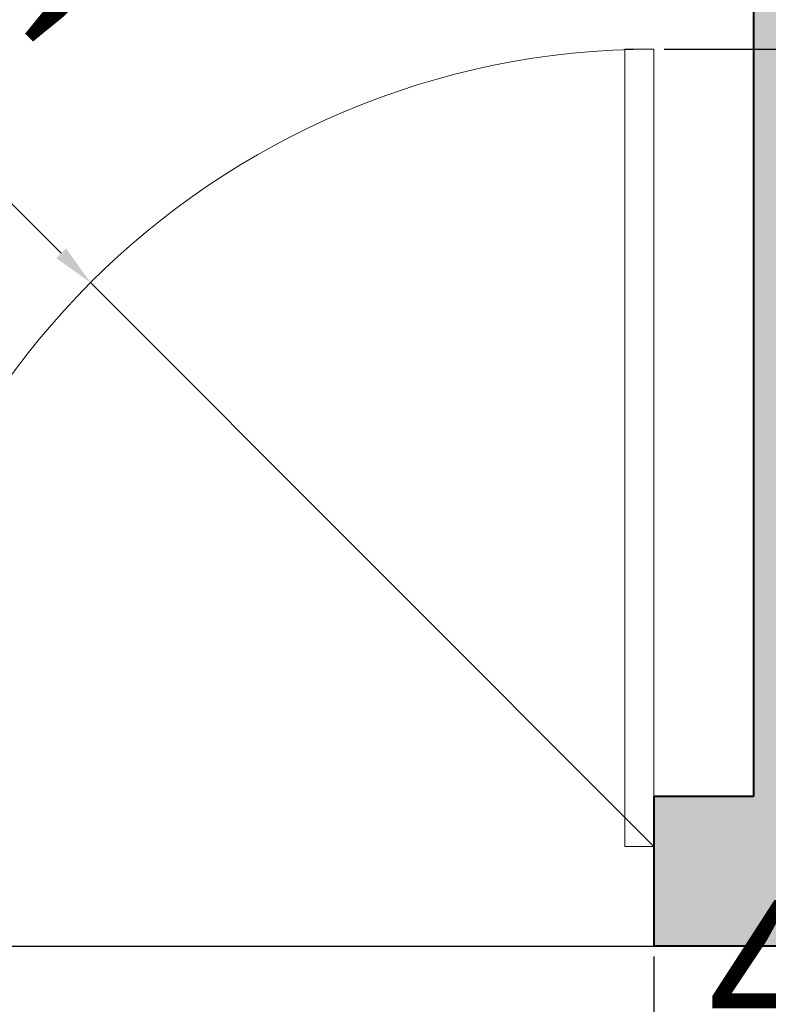
# Model space of a CAD drawing. Units: inches. Extents: x 2337 to 3570, y 1258 to 1938.
# Tile 24 of 30: x 3382 to 3427, y 1539 to 1598. Entities that reach past the tile are written whole.
import ezdxf

# ---------------------------------------------------------------- set-up
doc = ezdxf.new("R2010")
doc.units = ezdxf.units.IN
for name, color, linetype, lineweight in [('A-ANNO-DIMS', 2, 'Continuous', 18), ('A-DOOR', 4, 'Continuous', 20), ('A-WALL', 7, 'Continuous', 40)]:
    doc.layers.add(name, color=color, linetype=linetype, lineweight=lineweight)
doc.layers.add('A-WALL-PATT', color=18, linetype='Continuous', lineweight=13, true_color=0x000000)
doc.styles.get("Standard").update_dxf_attribs({"font": 'arial.ttf'})
doc.dimstyles.new('ISO-25', dxfattribs={"dimtxt": 9, "dimasz": 2.5, "dimexe": 1.25, "dimexo": 0.625, "dimtad": 1, "dimdec": 1, "dimlunit": 3, "dimtxsty": 'Standard', "dimcen": 2.5, "dimadec": 0, "dimazin": 0, "dimtfac": 1, "dimtdec": 1, "dimtmove": 0, "dimatfit": 3, "dimfxl": 1, "dimarcsym": 0})

# ---------------------------------------------------------------- blocks, each defined once
blk = doc.blocks.new('DOOR-SWING-48IN')
for p, q in [((0, 6), (0, 0)), ((48, 6), (48, 0))]:
    blk.add_line(p, q)
blk.add_lwpolyline([(48, 6), (48, 54), (46.25, 54), (46.25, 6)], close=True)
blk.add_arc((48, 6), 48, 90, 180)
blk = doc.blocks.new('*D68')
at = {"layer": 'A-ANNO-DIMS', "color": 0, "lineweight": -2, "transparency": 16777216}
for p, q in [((3427.886, 1596.116), (3427.886, 1741.994)), ((3420.411, 1596.116), (3429.136, 1596.116)), ((3427.886, 1544.616), (3427.886, 1593.616)), ((3420.411, 1542.116), (3429.136, 1542.116))]:
    blk.add_line(p, q, dxfattribs=at)
at = {"layer": 'A-ANNO-DIMS', "color": 0, "transparency": 16777216}
for points in [[(3427.469, 1593.616), (3428.303, 1593.616), (3427.886, 1596.116)], [(3427.469, 1544.616), (3428.303, 1544.616), (3427.886, 1542.116)]]:
    blk.add_solid(points, dxfattribs=at)
at = {"layer": 'Defpoints', "color": 0, "transparency": 16777216}
for p in [(3419.786, 1596.116), (3427.886, 1596.116), (3419.786, 1542.116)]:
    blk.add_point(p, dxfattribs=at)
at = {"layer": 'A-ANNO-DIMS', "color": 0, "transparency": 16777216, "insert": (3422.605, 1670.305), "char_height": 9, "attachment_point": 5, "rotation": 90}
blk.add_mtext('SWING DOOR 4\'-6" TYP.', dxfattribs=at)
blk = doc.blocks.new('*D69')
at = {"layer": 'A-ANNO-DIMS', "color": 0, "lineweight": -2, "transparency": 16777216}
for p, q in [((3371.786, 1541.491), (3371.786, 1532.766)), ((3419.786, 1541.491), (3419.786, 1532.766)), ((3374.286, 1534.016), (3417.286, 1534.016)), ((3419.786, 1534.016), (3478.758, 1534.016))]:
    blk.add_line(p, q, dxfattribs=at)
at = {"layer": 'A-ANNO-DIMS', "color": 0, "transparency": 16777216}
for points in [[(3374.286, 1534.433), (3374.286, 1533.599), (3371.786, 1534.016)], [(3417.286, 1534.433), (3417.286, 1533.599), (3419.786, 1534.016)]]:
    blk.add_solid(points, dxfattribs=at)
at = {"layer": 'Defpoints', "color": 0, "transparency": 16777216}
for p in [(3371.786, 1542.116), (3419.786, 1542.116), (3419.786, 1534.016)]:
    blk.add_point(p, dxfattribs=at)
at = {"layer": 'A-ANNO-DIMS', "color": 0, "transparency": 16777216, "insert": (3450.522, 1539.236), "char_height": 9, "attachment_point": 5}
blk.add_mtext('4\'-0" TYP.', dxfattribs=at)
blk = doc.blocks.new('*D115')
at = {"layer": 'A-ANNO-DIMS', "color": 0, "lineweight": -2, "transparency": 16777216}
for p, q in [((3243.411, 1542.116), (3502.436, 1542.116)), ((3501.186, 1539.616), (3501.186, 1526.616)), ((3243.411, 1524.116), (3502.436, 1524.116)), ((3501.186, 1524.116), (3501.186, 1497.289))]:
    blk.add_line(p, q, dxfattribs=at)
at = {"layer": 'A-ANNO-DIMS', "color": 0, "transparency": 16777216}
for points in [[(3500.769, 1539.616), (3501.603, 1539.616), (3501.186, 1542.116)], [(3500.769, 1526.616), (3501.603, 1526.616), (3501.186, 1524.116)]]:
    blk.add_solid(points, dxfattribs=at)
at = {"layer": 'Defpoints', "color": 0, "transparency": 16777216}
for p in [(3242.786, 1542.116), (3242.786, 1524.116), (3501.186, 1524.116)]:
    blk.add_point(p, dxfattribs=at)
at = {"layer": 'A-ANNO-DIMS', "color": 0, "transparency": 16777216, "insert": (3495.966, 1509.452), "char_height": 9, "attachment_point": 5, "rotation": 90}
blk.add_mtext('1\'-6"', dxfattribs=at)
blk = doc.blocks.new('*D120')
at = {"layer": 'A-ANNO-DIMS', "color": 0, "lineweight": -2, "transparency": 16777216}
for p, q in [((3353.535, 1614.367), (3384.077, 1583.825)), ((3419.786, 1548.116), (3385.845, 1582.057))]:
    blk.add_line(p, q, dxfattribs=at)
at = {"layer": 'A-ANNO-DIMS', "color": 0, "transparency": 16777216}
blk.add_solid([(3384.372, 1584.119), (3383.783, 1583.53), (3385.845, 1582.057)], dxfattribs=at)
at = {"layer": 'Defpoints', "color": 0, "transparency": 16777216}
for p in [(3385.845, 1582.057), (3419.786, 1548.116)]:
    blk.add_point(p, dxfattribs=at)
at = {"layer": 'A-ANNO-DIMS', "color": 0, "transparency": 16777216, "insert": (3369.171, 1606.113), "char_height": 9, "attachment_point": 5, "rotation": 315.0001}
blk.add_mtext('R4\'-0"', dxfattribs=at)

msp = doc.modelspace()

# ---------------------------------------------------------------- hatches: boundary and pattern name
at = {"layer": 'A-WALL-PATT'}
h = msp.add_hatch(color=256, dxfattribs=at)
h.dxf.hatch_style = 1
h.paths.add_polyline_path([(3233.786, 1857.116), (3017.786, 1857.116), (3017.786, 1824.116), (3026.786, 1824.116), (3026.786, 1848.116), (3233.786, 1848.116)])
h.paths.add_polyline_path([(3128.786, 1764.116), (3026.786, 1764.116), (3026.786, 1788.116), (3017.786, 1788.116), (3017.786, 1743.116), (3026.786, 1743.116), (3026.786, 1755.116), (3128.786, 1755.116)])
h.paths.add_polyline_path([(3245.786, 1761.116), (3245.786, 1764.116), (3164.786, 1764.116), (3164.786, 1755.116), (3170.786, 1755.116), (3170.786, 1701.116), (3224.786, 1701.116), (3224.786, 1605.116), (3233.786, 1605.116), (3233.786, 1713.116), (3224.786, 1713.116), (3224.786, 1707.116), (3176.786, 1707.116), (3176.786, 1755.116), (3224.786, 1755.116), (3224.786, 1749.116), (3233.786, 1749.116), (3233.786, 1755.116), (3245.786, 1755.116)])
h.paths.add_polyline_path([(3026.786, 1707.116), (3017.786, 1707.116), (3017.786, 1617.116), (3026.786, 1617.116), (3026.786, 1635.116), (3068.786, 1635.116), (3068.786, 1641.116), (3026.786, 1641.116)])
h.paths.add_polyline_path([(3104.786, 1551.116), (3026.786, 1551.116), (3026.786, 1569.116), (3017.786, 1569.116), (3017.786, 1518.116), (3026.786, 1518.116), (3026.786, 1542.116), (3104.786, 1542.116)])
h.paths.add_polyline_path([(3026.786, 1482.116), (3017.786, 1482.116), (3017.786, 1410.116), (3026.786, 1410.116)])
h.paths.add_polyline_path([(3188.786, 1350.116), (3152.786, 1350.116), (3152.786, 1380.116), (3146.786, 1380.116), (3146.786, 1350.116), (3026.786, 1350.116), (3026.786, 1374.116), (3017.786, 1374.116), (3017.786, 1341.116), (3188.786, 1341.116)])
h.paths.add_polyline_path([(3224.786, 1416.116), (3248.786, 1416.116), (3248.786, 1422.116), (3152.786, 1422.116), (3152.786, 1542.116), (3242.786, 1542.116), (3242.786, 1551.116), (3233.786, 1551.116), (3233.786, 1557.116), (3224.786, 1557.116), (3224.786, 1551.116), (3140.786, 1551.116), (3140.786, 1542.116), (3146.786, 1542.116), (3146.786, 1410.116), (3152.786, 1410.116), (3152.786, 1416.116), (3218.786, 1416.116), (3218.786, 1350.116), (3212.786, 1350.116), (3212.786, 1341.116), (3293.786, 1341.116), (3293.786, 1362.116), (3284.786, 1362.116), (3284.786, 1350.116), (3224.786, 1350.116)])
h.paths.add_polyline_path([(3293.786, 1434.116), (3284.786, 1434.116), (3284.786, 1422.116), (3278.786, 1422.116), (3278.786, 1416.116), (3284.786, 1416.116), (3284.786, 1386.116), (3293.786, 1386.116)], flags=17)
h.paths.add_polyline_path([(3293.786, 1542.116), (3314.786, 1542.116), (3314.786, 1551.116), (3278.786, 1551.116), (3278.786, 1545.116), (3278.786, 1542.116), (3284.786, 1542.116), (3284.786, 1482.116), (3293.786, 1482.116)])
h.paths.add_polyline_path([(3371.786, 1551.116), (3350.786, 1551.116), (3350.786, 1542.116), (3371.786, 1542.116), (3371.786, 1548.116)])
h.paths.add_polyline_path([(3434.786, 1647.116), (3425.786, 1647.116), (3425.786, 1551.116), (3419.786, 1551.116), (3419.786, 1548.116), (3419.786, 1542.116), (3434.786, 1542.116)])
h.paths.add_polyline_path([(3434.786, 1764.116), (3389.786, 1764.116), (3389.786, 1755.116), (3425.786, 1755.116), (3425.786, 1719.116), (3434.786, 1719.116)])
h.paths.add_polyline_path([(3317.786, 1764.116), (3281.786, 1764.116), (3281.786, 1755.116), (3317.786, 1755.116)])

# ---------------------------------------------------------------- linework, layer by layer
at = {"layer": 'A-WALL'}
for p, q in [((3425.786, 1755.116), (3425.786, 1551.116)), ((3425.786, 1551.116), (3419.786, 1551.116)), ((3419.786, 1551.116), (3419.786, 1542.116)), ((3434.786, 1542.116), (3419.786, 1542.116))]:
    msp.add_line(p, q, dxfattribs=at)

# ---------------------------------------------------------------- block references
at = {"layer": 'A-DOOR'}
msp.add_blockref('DOOR-SWING-48IN', (3371.786, 1542.116), dxfattribs=at)

# ---------------------------------------------------------------- dimensions: what is measured, and where the dimension line sits
at = {"layer": 'A-ANNO-DIMS'}
dim = msp.add_linear_dim(base=(3427.886, 1596.116), p1=(3419.786, 1542.116), p2=(3419.786, 1596.116), angle=90, text='SWING DOOR <> TYP.', dimstyle='ISO-25', override={"dimdec": 1, "dimlfac": 1, "dimrnd": 0, "dimzin": 1, "dimdsep": 46, "dimlunit": 4, "dimfrac": 2}, dxfattribs=at)
dim.commit()
dim.dimension.update_dxf_attribs({"geometry": '*D68', "text_midpoint": (3422.605, 1670.305)})
dim = msp.add_radius_dim(center=(3419.786, 1548.116), mpoint=(3385.845, 1582.057), dimstyle='ISO-25', override={"dimdec": 1, "dimlfac": 1, "dimrnd": 0, "dimzin": 1, "dimdsep": 46, "dimlunit": 4, "dimfrac": 2}, dxfattribs=at)
dim.commit()
dim.dimension.update_dxf_attribs({"geometry": '*D120', "text_midpoint": (3365.48, 1602.422), "dimtype": 164})
dim = msp.add_linear_dim(base=(3419.786, 1534.016), p1=(3371.786, 1542.116), p2=(3419.786, 1542.116), text='<> TYP.', dimstyle='ISO-25', override={"dimdec": 1, "dimlfac": 1, "dimrnd": 0, "dimzin": 1, "dimdsep": 46, "dimlunit": 4, "dimfrac": 2}, dxfattribs=at)
dim.commit()
dim.dimension.update_dxf_attribs({"geometry": '*D69', "text_midpoint": (3450.522, 1539.236)})
dim = msp.add_linear_dim(base=(3501.186, 1524.116), p1=(3242.786, 1542.116), p2=(3242.786, 1524.116), angle=90, dimstyle='ISO-25', override={"dimdec": 1, "dimlfac": 1, "dimrnd": 0, "dimzin": 1, "dimdsep": 46, "dimlunit": 4, "dimfrac": 2}, dxfattribs=at)
dim.commit()
dim.dimension.update_dxf_attribs({"geometry": '*D115', "text_midpoint": (3495.966, 1509.452)})

doc.saveas('drawing.dxf')
